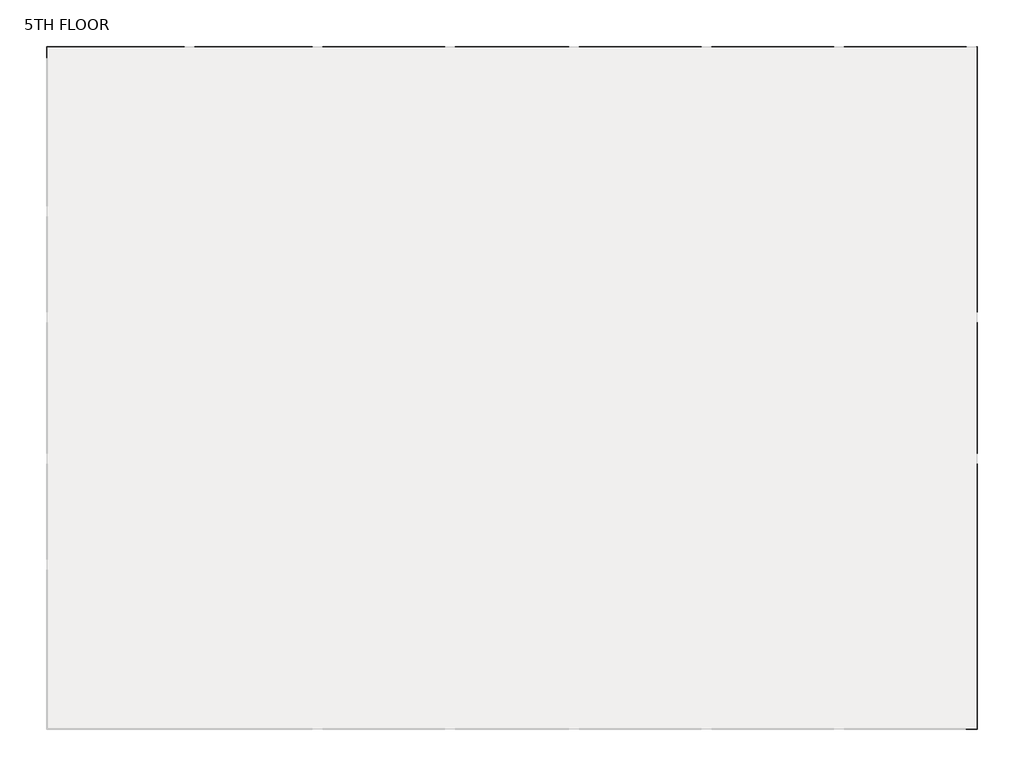
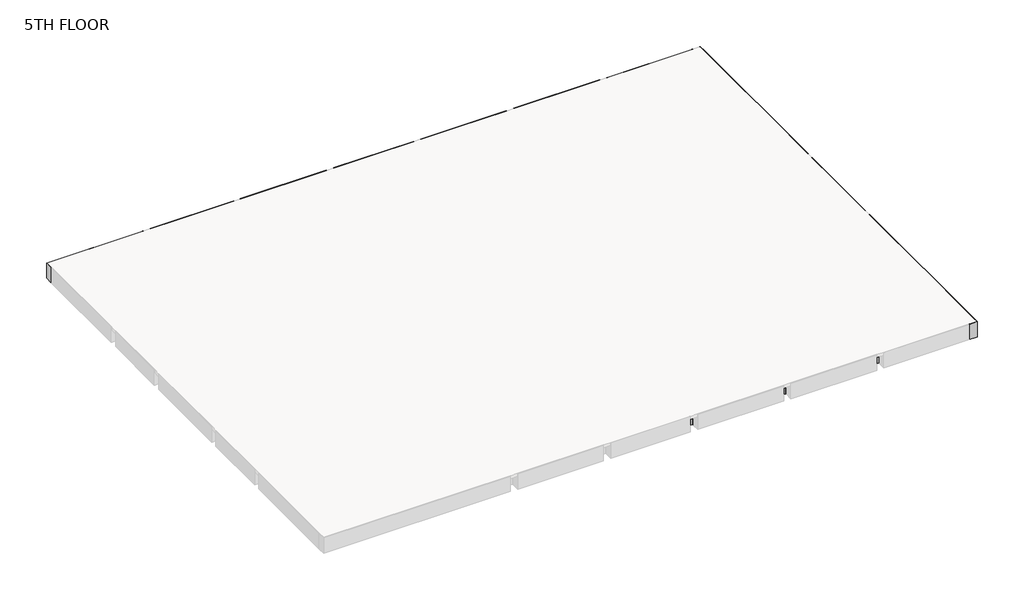
# One storey, part 2 of 2: 7 beams.
"""IFC4 building model written with IfcOpenShell, lengths in millimetres."""

from ifc_helpers import new_model, si_unit, frame, origin, place, context, project, spatial, polyline, outline, extrude, faceted_brep, element, save

model = new_model("IFC4")

# Units and contexts
model_context = context("Model", 3, world=origin())
ifc_project = project(units=[si_unit("LENGTHUNIT", "METRE", prefix="MILLI")], contexts=[model_context])

# Site, building, storey
site = spatial("IfcSite", under=ifc_project)
building = spatial("IfcBuilding", under=site)
storey = spatial("IfcBuildingStorey", under=building, Name="5TH FLOOR", Elevation=16764.0)

# Beams
placement = place(None, origin())
element("IfcBeam", 1, ObjectType="M_Concrete-Rectangular Beam : 400 x 800mm", at=placement, inside=storey, context=model_context, shape_type="Brep", body=[
    faceted_brep([(6397.6508981, 16716.9690835, 16764.0), (6397.6508981, 17116.9690835, 16764.0), (6375.4508981, 17116.9690835, 16764.0), (6375.4508981, 17094.7690835, 16764.0), (6375.4508981, 16716.9690835, 16764.0), (6397.6508981, 16716.9690835, 15964.0), (6375.4508981, 16716.9690835, 16611.6), (5997.6508981, 16716.9690835, 16611.6), (1825.6508981, 16716.9690835, 16611.6), (1803.4508981, 16716.9690835, 16611.6), (1803.4508981, 16716.9690835, 15964.0), (1825.6508981, 16716.9690835, 15964.0), (5997.6508981, 16716.9690835, 15964.0), (6397.6508981, 17116.9690835, 15964.0), (1803.4508981, 17116.9690835, 15964.0), (6019.8508981, 17116.9690835, 15964.0), (6019.8508981, 16789.9690835, 15964.0), (6375.4508981, 16789.9690835, 15964.0), (6375.4508981, 17116.9690835, 15964.0), (1803.4508981, 17094.7690835, 16611.6), (6019.8508981, 17094.7690835, 16611.6), (6019.8508981, 17094.7690835, 16764.0), (1803.4508981, 17094.7690835, 16764.0), (6375.4508981, 16789.9690835, 16611.6), (6019.8508981, 16789.9690835, 16611.6), (6019.8508981, 17116.9690835, 16764.0), (1803.4508981, 17116.9690835, 16764.0)], [[[0, 1, 2, 3, 4]], [[5, 0, 4, 6, 7, 8, 9, 10, 11, 12]], [[13, 5, 12, 11, 10, 14, 15, 16, 17, 18]], [[1, 13, 18, 2]], [[1, 0, 5, 13]], [[19, 20, 21, 22]], [[18, 17, 23, 6, 4, 3, 2]], [[17, 16, 24, 23]], [[16, 15, 25, 21, 20, 24]], [[25, 15, 14, 26]], [[14, 10, 9, 19, 22, 26]], [[20, 19, 9, 8, 7, 6, 23, 24]], [[25, 26, 22, 21]]]),
    faceted_brep([(-25701.5491019, 16716.9690835, 16764.0), (-25701.5491019, 17116.9690835, 16764.0), (-25701.5491019, 17116.9690835, 15964.0), (-25701.5491019, 16716.9690835, 15964.0), (-25323.7491019, 17094.7690835, 15964.0), (-25323.7491019, 16739.1690835, 15964.0), (-25323.7491019, 16739.1690835, 16611.6), (-25323.7491019, 17094.7690835, 16611.6), (-25679.3491019, 16739.1690835, 15964.0), (-25679.3491019, 16739.1690835, 16611.6), (-25679.3491019, 16716.9690835, 16764.0), (-25679.3491019, 16716.9690835, 16611.6), (-25679.3491019, 17094.7690835, 15964.0), (-25679.3491019, 17094.7690835, 16611.6), (-25679.3491019, 17094.7690835, 16764.0), (-20954.9491019, 16716.9690835, 15964.0), (-20954.9491019, 17116.9690835, 15964.0), (-20954.9491019, 17116.9690835, 16764.0), (-20954.9491019, 17094.7690835, 16764.0), (-20954.9491019, 17094.7690835, 16611.6), (-20954.9491019, 16716.9690835, 16611.6), (-25301.5491019, 16716.9690835, 15964.0), (-20977.1491019, 16716.9690835, 15964.0), (-20977.1491019, 16716.9690835, 16611.6), (-25301.5491019, 16716.9690835, 16611.6)], [[[0, 1, 2, 3]], [[4, 5, 6, 7]], [[5, 8, 9, 6]], [[10, 11, 9, 8, 12, 13, 14]], [[15, 16, 17, 18, 19, 20]], [[1, 0, 10, 14, 18, 17]], [[0, 3, 21, 22, 15, 20, 23, 24, 11, 10]], [[3, 2, 16, 15, 22, 21], [5, 4, 12, 8]], [[2, 1, 17, 16]], [[14, 13, 12, 4, 7, 19, 18]], [[19, 7, 6, 9, 11, 24, 23, 20]]]),
    faceted_brep([(-16179.7491019, 17116.9690835, 15964.0), (-16179.7491019, 16716.9690835, 15964.0), (-16179.7491019, 16716.9690835, 16611.6), (-16179.7491019, 17094.7690835, 16611.6), (-16179.7491019, 17094.7690835, 16764.0), (-16179.7491019, 17116.9690835, 16764.0), (-11963.3491019, 16716.9690835, 15964.0), (-11963.3491019, 17116.9690835, 15964.0), (-11963.3491019, 17116.9690835, 16764.0), (-11963.3491019, 17094.7690835, 16764.0), (-11963.3491019, 17094.7690835, 16611.6), (-11963.3491019, 16716.9690835, 16611.6), (-16157.5491019, 16716.9690835, 15964.0), (-11985.5491019, 16716.9690835, 15964.0), (-11985.5491019, 16716.9690835, 16611.6), (-16157.5491019, 16716.9690835, 16611.6)], [[[0, 1, 2, 3, 4, 5]], [[6, 7, 8, 9, 10, 11]], [[8, 5, 4, 9]], [[1, 12, 13, 6, 11, 14, 15, 2]], [[1, 0, 7, 6, 13, 12]], [[0, 5, 8, 7]], [[3, 10, 9, 4]], [[10, 3, 2, 15, 14, 11]]]),
    faceted_brep([(-16535.3491019, 16716.9690835, 15964.0), (-16535.3491019, 17116.9690835, 15964.0), (-16535.3491019, 17116.9690835, 16764.0), (-16535.3491019, 17094.7690835, 16764.0), (-16535.3491019, 17094.7690835, 16611.6), (-16535.3491019, 16716.9690835, 16611.6), (-20599.3491019, 17116.9690835, 16764.0), (-20599.3491019, 17094.7690835, 16764.0), (-20599.3491019, 16716.9690835, 15964.0), (-20577.1491019, 16716.9690835, 15964.0), (-16557.5491019, 16716.9690835, 15964.0), (-16557.5491019, 16716.9690835, 16611.6), (-20577.1491019, 16716.9690835, 16611.6), (-20599.3491019, 16716.9690835, 16611.6), (-20599.3491019, 17116.9690835, 15964.0), (-20599.3491019, 17094.7690835, 16611.6)], [[[0, 1, 2, 3, 4, 5]], [[2, 6, 7, 3]], [[8, 9, 10, 0, 5, 11, 12, 13]], [[1, 0, 10, 9, 8, 14]], [[2, 1, 14, 6]], [[14, 8, 13, 15, 7, 6]], [[15, 4, 3, 7]], [[4, 15, 13, 12, 11, 5]]]),
    faceted_brep([(-11607.7491019, 17116.9690835, 15964.0), (-11607.7491019, 16716.9690835, 15964.0), (-11607.7491019, 16716.9690835, 16611.6), (-11607.7491019, 17094.7690835, 16611.6), (-11607.7491019, 17094.7690835, 16764.0), (-11607.7491019, 17116.9690835, 16764.0), (-7696.1491019, 16716.9690835, 15964.0), (-7696.1491019, 17116.9690835, 15964.0), (-7696.1491019, 17116.9690835, 16764.0), (-7696.1491019, 17094.7690835, 16764.0), (-7696.1491019, 17094.7690835, 16611.6), (-7696.1491019, 16716.9690835, 16611.6), (-11585.5491019, 16716.9690835, 15964.0), (-7718.3491019, 16716.9690835, 15964.0), (-7718.3491019, 16716.9690835, 16611.6), (-11585.5491019, 16716.9690835, 16611.6)], [[[0, 1, 2, 3, 4, 5]], [[6, 7, 8, 9, 10, 11]], [[8, 5, 4, 9]], [[1, 12, 13, 6, 11, 14, 15, 2]], [[1, 0, 7, 6, 13, 12]], [[0, 5, 8, 7]], [[3, 10, 9, 4]], [[10, 3, 2, 15, 14, 11]]]),
    faceted_brep([(-7340.5491019, 17116.9690835, 15964.0), (-7340.5491019, 16716.9690835, 15964.0), (-7340.5491019, 16716.9690835, 16611.6), (-7340.5491019, 17094.7690835, 16611.6), (-7340.5491019, 17094.7690835, 16764.0), (-7340.5491019, 17116.9690835, 16764.0), (-3124.1491019, 16716.9690835, 15964.0), (-3124.1491019, 17116.9690835, 15964.0), (-3124.1491019, 17116.9690835, 16764.0), (-3124.1491019, 17094.7690835, 16764.0), (-3124.1491019, 17094.7690835, 16611.6), (-3124.1491019, 16716.9690835, 16611.6), (-7318.3491019, 16716.9690835, 15964.0), (-3146.3491019, 16716.9690835, 15964.0), (-3146.3491019, 16716.9690835, 16611.6), (-7318.3491019, 16716.9690835, 16611.6)], [[[0, 1, 2, 3, 4, 5]], [[6, 7, 8, 9, 10, 11]], [[8, 5, 4, 9]], [[1, 12, 13, 6, 11, 14, 15, 2]], [[1, 0, 7, 6, 13, 12]], [[0, 5, 8, 7]], [[3, 10, 9, 4]], [[10, 3, 2, 15, 14, 11]]]),
    faceted_brep([(-2768.5491019, 17116.9690835, 15964.0), (-2768.5491019, 16716.9690835, 15964.0), (-2768.5491019, 16716.9690835, 16611.6), (-2768.5491019, 17094.7690835, 16611.6), (-2768.5491019, 17094.7690835, 16764.0), (-2768.5491019, 17116.9690835, 16764.0), (1447.8508981, 16716.9690835, 15964.0), (1447.8508981, 17116.9690835, 15964.0), (1447.8508981, 17116.9690835, 16764.0), (1447.8508981, 17094.7690835, 16764.0), (1447.8508981, 17094.7690835, 16611.6), (1447.8508981, 16716.9690835, 16611.6), (-2746.3491019, 16716.9690835, 15964.0), (1425.6508981, 16716.9690835, 15964.0), (1425.6508981, 16716.9690835, 16611.6), (-2746.3491019, 16716.9690835, 16611.6)], [[[0, 1, 2, 3, 4, 5]], [[6, 7, 8, 9, 10, 11]], [[8, 5, 4, 9]], [[1, 12, 13, 6, 11, 14, 15, 2]], [[1, 0, 7, 6, 13, 12]], [[0, 5, 8, 7]], [[3, 10, 9, 4]], [[10, 3, 2, 15, 14, 11]]]),
])
element("IfcBeam", 2, ObjectType="M_Concrete-Rectangular Beam : 400 x 800mm", at=placement, inside=storey, context=model_context, shape_type="Brep", body=[
    faceted_brep([(5997.6508981, -6447.8309165, 16764.0), (6397.6508981, -6447.8309165, 16764.0), (6397.6508981, 2718.3690835, 16764.0), (6375.4508981, 2718.3690835, 16764.0), (6375.4508981, -507.4309165, 16764.0), (6375.4508981, -1015.4309165, 16764.0), (6375.4508981, -6425.6309165, 16764.0), (5997.6508981, -6425.6309165, 16764.0), (5997.6508981, -6447.8309165, 15964.0), (5997.6508981, -6425.6309165, 16611.6), (5997.6508981, -6047.8309165, 16611.6), (5997.6508981, -961.4309165, 16611.6), (5997.6508981, -561.4309165, 16611.6), (5997.6508981, 2696.1690835, 16611.6), (5997.6508981, 2718.3690835, 16611.6), (5997.6508981, 2718.3690835, 15964.0), (5997.6508981, 2696.1690835, 15964.0), (5997.6508981, -561.4309165, 15964.0), (5997.6508981, -961.4309165, 15964.0), (5997.6508981, -6047.8309165, 15964.0), (6397.6508981, -6447.8309165, 15964.0), (6397.6508981, 2718.3690835, 15964.0), (6375.4508981, -6425.6309165, 15964.0), (6375.4508981, -6070.0309165, 15964.0), (6019.8508981, -6070.0309165, 15964.0), (6019.8508981, -6425.6309165, 15964.0), (6375.4508981, -1015.4309165, 15964.0), (6375.4508981, -507.4309165, 15964.0), (6019.8508981, -507.4309165, 15964.0), (6019.8508981, -1015.4309165, 15964.0), (6375.4508981, 2718.3690835, 16611.6), (6375.4508981, -507.4309165, 16611.6), (6375.4508981, -1015.4309165, 16611.6), (6375.4508981, -6070.0309165, 16611.6), (6375.4508981, -6425.6309165, 16611.6), (6019.8508981, -6425.6309165, 16611.6), (6019.8508981, -6070.0309165, 16611.6), (6019.8508981, -1015.4309165, 16611.6), (6019.8508981, -507.4309165, 16611.6)], [[[0, 1, 2, 3, 4, 5, 6, 7]], [[8, 0, 7, 9, 10, 11, 12, 13, 14, 15, 16, 17, 18, 19]], [[20, 8, 19, 18, 17, 16, 15, 21], [22, 23, 24, 25], [26, 27, 28, 29]], [[1, 20, 21, 2]], [[1, 0, 8, 20]], [[3, 30, 31, 27, 26, 32, 33, 23, 22, 34, 6, 5, 4]], [[6, 34, 22, 25, 35, 9, 7]], [[25, 24, 36, 35]], [[24, 23, 33, 36]], [[21, 15, 14, 30, 3, 2]], [[26, 29, 37, 32]], [[29, 28, 38, 37]], [[28, 27, 31, 38]], [[33, 32, 37, 38, 31, 30, 14, 13, 12, 11, 10, 9, 35, 36]]]),
    faceted_brep([(6397.6508981, 16716.9690835, 15964.0), (5997.6508981, 16716.9690835, 15964.0), (5997.6508981, 16716.9690835, 16611.6), (6375.4508981, 16716.9690835, 16611.6), (6375.4508981, 16716.9690835, 16764.0), (6397.6508981, 16716.9690835, 16764.0), (5997.6508981, 7950.7690835, 15964.0), (6397.6508981, 7950.7690835, 15964.0), (6397.6508981, 7950.7690835, 16764.0), (6375.4508981, 7950.7690835, 16764.0), (6375.4508981, 7950.7690835, 16611.6), (5997.6508981, 7950.7690835, 16611.6), (6375.4508981, 11684.5690835, 16764.0), (6375.4508981, 11176.5690835, 16764.0), (5997.6508981, 11630.5690835, 15964.0), (5997.6508981, 11230.5690835, 15964.0), (5997.6508981, 7972.9690835, 15964.0), (5997.6508981, 7972.9690835, 16611.6), (5997.6508981, 11230.5690835, 16611.6), (5997.6508981, 11630.5690835, 16611.6), (6375.4508981, 11176.5690835, 15964.0), (6375.4508981, 11684.5690835, 15964.0), (6019.8508981, 11684.5690835, 15964.0), (6019.8508981, 11176.5690835, 15964.0), (6019.8508981, 11176.5690835, 16611.6), (6375.4508981, 11176.5690835, 16611.6), (6019.8508981, 11684.5690835, 16611.6), (6375.4508981, 11684.5690835, 16611.6)], [[[0, 1, 2, 3, 4, 5]], [[6, 7, 8, 9, 10, 11]], [[8, 5, 4, 12, 13, 9]], [[1, 14, 15, 16, 6, 11, 17, 18, 19, 2]], [[1, 0, 7, 6, 16, 15, 14], [20, 21, 22, 23]], [[0, 5, 8, 7]], [[20, 23, 24, 25]], [[23, 22, 26, 24]], [[22, 21, 27, 26]], [[27, 3, 2, 19, 18, 17, 11, 10, 25, 24, 26]], [[25, 10, 9, 13, 12, 4, 3, 27, 21, 20]]]),
    faceted_brep([(6397.6508981, 7595.1690835, 15964.0), (5997.6508981, 7595.1690835, 15964.0), (5997.6508981, 7595.1690835, 16611.6), (6375.4508981, 7595.1690835, 16611.6), (6375.4508981, 7595.1690835, 16764.0), (6397.6508981, 7595.1690835, 16764.0), (5997.6508981, 3073.9690835, 15964.0), (6397.6508981, 3073.9690835, 15964.0), (6397.6508981, 3073.9690835, 16764.0), (6375.4508981, 3073.9690835, 16764.0), (6375.4508981, 3073.9690835, 16611.6), (5997.6508981, 3073.9690835, 16611.6), (5997.6508981, 7572.9690835, 15964.0), (5997.6508981, 3096.1690835, 15964.0), (5997.6508981, 3096.1690835, 16611.6), (5997.6508981, 7572.9690835, 16611.6)], [[[0, 1, 2, 3, 4, 5]], [[6, 7, 8, 9, 10, 11]], [[8, 5, 4, 9]], [[1, 12, 13, 6, 11, 14, 15, 2]], [[1, 0, 7, 6, 13, 12]], [[0, 5, 8, 7]], [[3, 10, 9, 4]], [[10, 3, 2, 15, 14, 11]]]),
])
element("IfcBeam", 3, ObjectType="M_Concrete-Rectangular Beam : 400 x 800mm", at=placement, inside=storey, context=model_context, shape_type="SweptSolid", body=[
    extrude(outline(polyline([(-7318.3491019, -6047.8309165), (-7340.5491019, -6047.8309165), (-7340.5491019, -6019.2309165), (-7696.1491019, -6019.2309165), (-7696.1491019, -6047.8309165), (-7718.3491019, -6047.8309165), (-7718.3491019, -990.0309165), (-7318.3491019, -990.0309165), (-7318.3491019, -6047.8309165)])), frame((0.0, 0.0, 15964.0), z_axis=(0.0, 0.0, 1.0), x_axis=(1.0, 0.0, 0.0)), (0.0, 0.0, 1.0), 647.6),
    extrude(outline(polyline([(-7340.5491019, 16716.9690835), (-7318.3491019, 16716.9690835), (-7318.3491019, 11659.1690835), (-7718.3491019, 11659.1690835), (-7718.3491019, 16716.9690835), (-7696.1491019, 16716.9690835), (-7696.1491019, 16688.3690835), (-7340.5491019, 16688.3690835), (-7340.5491019, 16716.9690835)])), frame((0.0, 0.0, 15964.0), z_axis=(0.0, 0.0, 1.0), x_axis=(1.0, 0.0, 0.0)), (0.0, 0.0, 1.0), 647.6),
    extrude(outline(polyline([(-7718.3491019, 7544.3690835), (-7318.3491019, 7544.3690835), (-7318.3491019, 3124.7690835), (-7718.3491019, 3124.7690835), (-7718.3491019, 7544.3690835)])), frame((0.0, 0.0, 15964.0), z_axis=(0.0, 0.0, 1.0), x_axis=(1.0, 0.0, 0.0)), (0.0, 0.0, 1.0), 647.6),
    extrude(outline(polyline([(-7318.3491019, 8001.5690835), (-7718.3491019, 8001.5690835), (-7718.3491019, 11201.9690835), (-7318.3491019, 11201.9690835), (-7318.3491019, 8001.5690835)])), frame((0.0, 0.0, 15964.0), z_axis=(0.0, 0.0, 1.0), x_axis=(1.0, 0.0, 0.0)), (0.0, 0.0, 1.0), 647.6),
    extrude(outline(polyline([(-7318.3491019, -532.8309165), (-7718.3491019, -532.8309165), (-7718.3491019, 2667.5690835), (-7318.3491019, 2667.5690835), (-7318.3491019, -532.8309165)])), frame((0.0, 0.0, 15964.0), z_axis=(0.0, 0.0, 1.0), x_axis=(1.0, 0.0, 0.0)), (0.0, 0.0, 1.0), 647.6),
])
element("IfcBeam", 4, ObjectType="M_Concrete-Rectangular Beam : 400 x 800mm", at=placement, inside=storey, context=model_context, shape_type="SweptSolid", body=[
    extrude(outline(polyline([(-2746.3491019, -6047.8309165), (-2768.5491019, -6047.8309165), (-2768.5491019, -6019.2309165), (-3124.1491019, -6019.2309165), (-3124.1491019, -6047.8309165), (-3146.3491019, -6047.8309165), (-3146.3491019, -990.0309165), (-2746.3491019, -990.0309165), (-2746.3491019, -6047.8309165)])), frame((0.0, 0.0, 15964.0), z_axis=(0.0, 0.0, 1.0), x_axis=(1.0, 0.0, 0.0)), (0.0, 0.0, 1.0), 647.6),
    extrude(outline(polyline([(-2768.5491019, 16716.9690835), (-2746.3491019, 16716.9690835), (-2746.3491019, 11659.1690835), (-3146.3491019, 11659.1690835), (-3146.3491019, 16716.9690835), (-3124.1491019, 16716.9690835), (-3124.1491019, 16688.3690835), (-2768.5491019, 16688.3690835), (-2768.5491019, 16716.9690835)])), frame((0.0, 0.0, 15964.0), z_axis=(0.0, 0.0, 1.0), x_axis=(1.0, 0.0, 0.0)), (0.0, 0.0, 1.0), 647.6),
    extrude(outline(polyline([(-3146.3491019, 11201.9690835), (-2746.3491019, 11201.9690835), (-2746.3491019, 8001.5690835), (-3146.3491019, 8001.5690835), (-3146.3491019, 11201.9690835)])), frame((0.0, 0.0, 15964.0), z_axis=(0.0, 0.0, 1.0), x_axis=(1.0, 0.0, 0.0)), (0.0, 0.0, 1.0), 647.6),
    extrude(outline(polyline([(-3146.3491019, 7544.3690835), (-2746.3491019, 7544.3690835), (-2746.3491019, 3124.7690835), (-3146.3491019, 3124.7690835), (-3146.3491019, 7544.3690835)])), frame((0.0, 0.0, 15964.0), z_axis=(0.0, 0.0, 1.0), x_axis=(1.0, 0.0, 0.0)), (0.0, 0.0, 1.0), 647.6),
    extrude(outline(polyline([(-2746.3491019, -532.8309165), (-3146.3491019, -532.8309165), (-3146.3491019, 2667.5690835), (-2746.3491019, 2667.5690835), (-2746.3491019, -532.8309165)])), frame((0.0, 0.0, 15964.0), z_axis=(0.0, 0.0, 1.0), x_axis=(1.0, 0.0, 0.0)), (0.0, 0.0, 1.0), 647.6),
])
element("IfcBeam", 5, ObjectType="M_Concrete-Rectangular Beam : 400 x 800mm", at=placement, inside=storey, context=model_context, shape_type="SweptSolid", body=[
    extrude(outline(polyline([(1825.6508981, -6047.8309165), (1803.4508981, -6047.8309165), (1803.4508981, -6019.2309165), (1447.8508981, -6019.2309165), (1447.8508981, -6047.8309165), (1425.6508981, -6047.8309165), (1425.6508981, -990.0309165), (1825.6508981, -990.0309165), (1825.6508981, -6047.8309165)])), frame((0.0, 0.0, 15964.0), z_axis=(0.0, 0.0, 1.0), x_axis=(1.0, 0.0, 0.0)), (0.0, 0.0, 1.0), 647.6),
    extrude(outline(polyline([(1803.4508981, 16716.9690835), (1825.6508981, 16716.9690835), (1825.6508981, 11659.1690835), (1425.6508981, 11659.1690835), (1425.6508981, 16716.9690835), (1447.8508981, 16716.9690835), (1447.8508981, 16713.7690835), (1803.4508981, 16713.7690835), (1803.4508981, 16716.9690835)])), frame((0.0, 0.0, 15964.0), z_axis=(0.0, 0.0, 1.0), x_axis=(1.0, 0.0, 0.0)), (0.0, 0.0, 1.0), 647.6),
    extrude(outline(polyline([(1425.6508981, 11201.9690835), (1825.6508981, 11201.9690835), (1825.6508981, 8001.5690835), (1425.6508981, 8001.5690835), (1425.6508981, 11201.9690835)])), frame((0.0, 0.0, 15964.0), z_axis=(0.0, 0.0, 1.0), x_axis=(1.0, 0.0, 0.0)), (0.0, 0.0, 1.0), 647.6),
    extrude(outline(polyline([(1425.6508981, 7544.3690835), (1825.6508981, 7544.3690835), (1825.6508981, 3124.7690835), (1425.6508981, 3124.7690835), (1425.6508981, 7544.3690835)])), frame((0.0, 0.0, 15964.0), z_axis=(0.0, 0.0, 1.0), x_axis=(1.0, 0.0, 0.0)), (0.0, 0.0, 1.0), 647.6),
    extrude(outline(polyline([(1825.6508981, -532.8309165), (1425.6508981, -532.8309165), (1425.6508981, 2667.5690835), (1825.6508981, 2667.5690835), (1825.6508981, -532.8309165)])), frame((0.0, 0.0, 15964.0), z_axis=(0.0, 0.0, 1.0), x_axis=(1.0, 0.0, 0.0)), (0.0, 0.0, 1.0), 647.6),
])
element("IfcBeam", 6, ObjectType="M_Concrete-Rectangular Beam : 400 x 800mm", at=placement, inside=storey, context=model_context, shape_type="SweptSolid", body=[
    extrude(outline(polyline([(-25301.5491019, 11608.3690835), (-25301.5491019, 11630.5690835), (-21005.7491019, 11630.5690835), (-21005.7491019, 11230.5690835), (-25301.5491019, 11230.5690835), (-25301.5491019, 11252.7690835), (-25247.5491019, 11252.7690835), (-25247.5491019, 11608.3690835), (-25301.5491019, 11608.3690835)])), frame((0.0, 0.0, 15964.0), z_axis=(0.0, 0.0, 1.0), x_axis=(1.0, 0.0, 0.0)), (0.0, 0.0, 1.0), 647.6),
    extrude(outline(polyline([(5997.6508981, 11630.5690835), (5997.6508981, 11230.5690835), (1854.2508981, 11230.5690835), (1854.2508981, 11630.5690835), (5997.6508981, 11630.5690835)])), frame((0.0, 0.0, 15964.0), z_axis=(0.0, 0.0, 1.0), x_axis=(1.0, 0.0, 0.0)), (0.0, 0.0, 1.0), 647.6),
    extrude(outline(polyline([(-20548.5491019, 11230.5690835), (-20548.5491019, 11630.5690835), (-16586.1491019, 11630.5690835), (-16586.1491019, 11230.5690835), (-20548.5491019, 11230.5690835)])), frame((0.0, 0.0, 15964.0), z_axis=(0.0, 0.0, 1.0), x_axis=(1.0, 0.0, 0.0)), (0.0, 0.0, 1.0), 647.6),
    extrude(outline(polyline([(-16128.9491019, 11230.5690835), (-16128.9491019, 11630.5690835), (-12014.1491019, 11630.5690835), (-12014.1491019, 11230.5690835), (-16128.9491019, 11230.5690835)])), frame((0.0, 0.0, 15964.0), z_axis=(0.0, 0.0, 1.0), x_axis=(1.0, 0.0, 0.0)), (0.0, 0.0, 1.0), 647.6),
    extrude(outline(polyline([(-11556.9491019, 11230.5690835), (-11556.9491019, 11630.5690835), (-7746.9491019, 11630.5690835), (-7746.9491019, 11230.5690835), (-11556.9491019, 11230.5690835)])), frame((0.0, 0.0, 15964.0), z_axis=(0.0, 0.0, 1.0), x_axis=(1.0, 0.0, 0.0)), (0.0, 0.0, 1.0), 647.6),
    extrude(outline(polyline([(-7289.7491019, 11230.5690835), (-7289.7491019, 11630.5690835), (-3174.9491019, 11630.5690835), (-3174.9491019, 11230.5690835), (-7289.7491019, 11230.5690835)])), frame((0.0, 0.0, 15964.0), z_axis=(0.0, 0.0, 1.0), x_axis=(1.0, 0.0, 0.0)), (0.0, 0.0, 1.0), 647.6),
    extrude(outline(polyline([(-2717.7491019, 11230.5690835), (-2717.7491019, 11630.5690835), (1397.0508981, 11630.5690835), (1397.0508981, 11230.5690835), (-2717.7491019, 11230.5690835)])), frame((0.0, 0.0, 15964.0), z_axis=(0.0, 0.0, 1.0), x_axis=(1.0, 0.0, 0.0)), (0.0, 0.0, 1.0), 647.6),
])
element("IfcBeam", 7, ObjectType="M_Concrete-Rectangular Beam : 400 x 800mm", at=placement, inside=storey, context=model_context, shape_type="SweptSolid", body=[
    extrude(outline(polyline([(-25301.5491019, 7950.7690835), (-25301.5491019, 7972.9690835), (-21005.7491019, 7972.9690835), (-21005.7491019, 7572.9690835), (-25301.5491019, 7572.9690835), (-25301.5491019, 7595.1690835), (-25272.9491019, 7595.1690835), (-25272.9491019, 7950.7690835), (-25301.5491019, 7950.7690835)])), frame((0.0, 0.0, 15964.0), z_axis=(0.0, 0.0, 1.0), x_axis=(1.0, 0.0, 0.0)), (0.0, 0.0, 1.0), 647.6),
    extrude(outline(polyline([(5997.6508981, 7972.9690835), (5997.6508981, 7950.7690835), (5969.0508981, 7950.7690835), (5969.0508981, 7595.1690835), (5997.6508981, 7595.1690835), (5997.6508981, 7572.9690835), (1854.2508981, 7572.9690835), (1854.2508981, 7972.9690835), (5997.6508981, 7972.9690835)])), frame((0.0, 0.0, 15964.0), z_axis=(0.0, 0.0, 1.0), x_axis=(1.0, 0.0, 0.0)), (0.0, 0.0, 1.0), 647.6),
    extrude(outline(polyline([(-7289.7491019, 7572.9690835), (-7289.7491019, 7972.9690835), (-3174.9491019, 7972.9690835), (-3174.9491019, 7572.9690835), (-7289.7491019, 7572.9690835)])), frame((0.0, 0.0, 15964.0), z_axis=(0.0, 0.0, 1.0), x_axis=(1.0, 0.0, 0.0)), (0.0, 0.0, 1.0), 647.6),
    extrude(outline(polyline([(-7746.9491019, 7972.9690835), (-7746.9491019, 7572.9690835), (-11556.9491019, 7572.9690835), (-11556.9491019, 7972.9690835), (-7746.9491019, 7972.9690835)])), frame((0.0, 0.0, 15964.0), z_axis=(0.0, 0.0, 1.0), x_axis=(1.0, 0.0, 0.0)), (0.0, 0.0, 1.0), 647.6),
    extrude(outline(polyline([(1397.0508981, 7972.9690835), (1397.0508981, 7572.9690835), (-2717.7491019, 7572.9690835), (-2717.7491019, 7972.9690835), (1397.0508981, 7972.9690835)])), frame((0.0, 0.0, 15964.0), z_axis=(0.0, 0.0, 1.0), x_axis=(1.0, 0.0, 0.0)), (0.0, 0.0, 1.0), 647.6),
    extrude(outline(polyline([(-12014.1491019, 7972.9690835), (-12014.1491019, 7572.9690835), (-16128.9491019, 7572.9690835), (-16128.9491019, 7972.9690835), (-12014.1491019, 7972.9690835)])), frame((0.0, 0.0, 15964.0), z_axis=(0.0, 0.0, 1.0), x_axis=(1.0, 0.0, 0.0)), (0.0, 0.0, 1.0), 647.6),
    extrude(outline(polyline([(-16586.1491019, 7972.9690835), (-16586.1491019, 7572.9690835), (-20548.5491019, 7572.9690835), (-20548.5491019, 7972.9690835), (-16586.1491019, 7972.9690835)])), frame((0.0, 0.0, 15964.0), z_axis=(0.0, 0.0, 1.0), x_axis=(1.0, 0.0, 0.0)), (0.0, 0.0, 1.0), 647.6),
])

save(model, "model.ifc")

# Revit data of these elements
# Type "M_Concrete-Rectangular Beam : 400 x 800mm"
#   Length [instance default] = 5' - 0"
#   b = 1' - 3.74803"
#   h = 2' - 7.49606"
#   Structural Material [instance default] = Concrete, Cast-in-Place gray
#   Assembly Code = ""
# Elements 1, 2 (IfcBeam, "M_Concrete-Rectangular Beam : 400 x 800mm")
#   Structural Material = Concrete, Cast-in-Place gray
#   Phase Created = New Construction
#   Materials on its faces: "Concrete, Cast-in-Place gray"
# Elements 3, 4, 5, 6, 7 (IfcBeam, "M_Concrete-Rectangular Beam : 400 x 800mm")
#   Comments = ""
#   Structural Material = Concrete, Cast-in-Place gray
#   Phase Created = New Construction
#   Materials on its faces: "Concrete, Cast-in-Place gray"
# Materials
#   "Concrete, Cast-in-Place gray": class "Concrete", colour RGB 192 192 192, transparency 0, Description = "Cast-in-place concrete", Cost = 0
